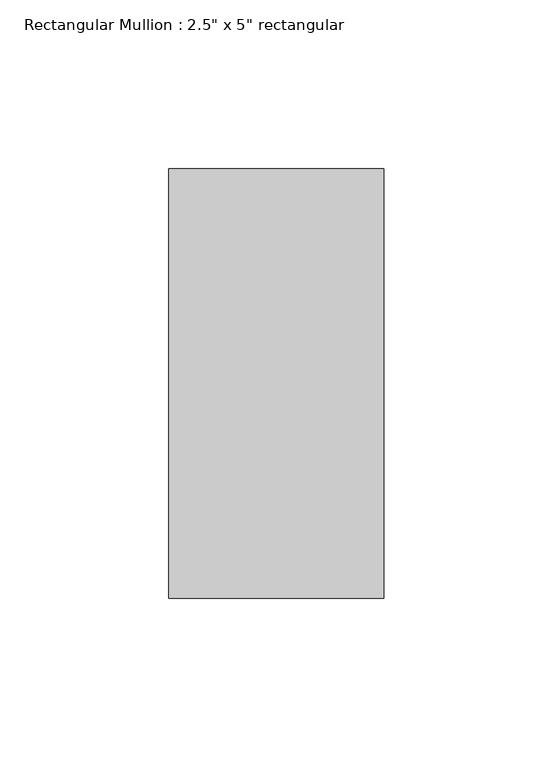
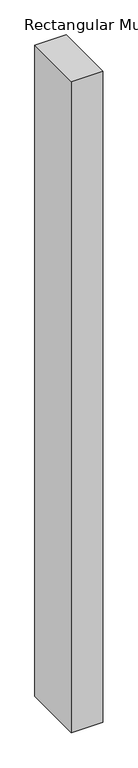
"""IFC4 building model written with IfcOpenShell, lengths in millimetres: member geometry."""

from ifc_helpers import new_model, si_unit, frame, origin, place, context, project, spatial, polyline, outline, extrude, source, transform, mapped, element, save


def member_331a33ef(model_context):
    return source(origin(), model_context, "Body", "SweptSolid", [
        extrude(outline(polyline([(0.0, 63.5), (0.0, -63.5), (-63.5, -63.5), (-63.5, 63.5), (0.0, 63.5)])), frame((0.0, 0.0, -1387.342808), z_axis=(0.0, 0.0, 1.0), x_axis=(1.0, 0.0, 0.0)), (0.0, 0.0, 1.0), 1387.342808),
    ])


if __name__ == "__main__":
    model = new_model("IFC4")
    model_context = context("Model", 3, world=origin())
    ifc_project = project(units=[si_unit("LENGTHUNIT", "METRE", prefix="MILLI")], contexts=[model_context])
    site = spatial("IfcSite", under=ifc_project)
    building = spatial("IfcBuilding", under=site)
    placement = place(None, origin())
    member_shape = member_331a33ef(model_context)
    element("IfcMember", 1, ObjectType="Rectangular Mullion : 2.5\" x 5\" rectangular", at=placement, inside=building, context=model_context, shape_type="MappedRepresentation", body=[
        mapped(member_shape, transform((0.0, 0.0, 0.0), x_axis=(1.0, 0.0, 0.0), y_axis=(0.0, 1.0, 0.0), z_axis=(0.0, 0.0, 1.0))),
    ])
    save(model, "model.ifc")

# Revit data of these elements
# Type "Rectangular Mullion : 2.5\" x 5\" rectangular"
#   built-in parameter 1007304 = 0.416667 (stored number, unit not read)
#   built-in parameter 1007301 = 0.104167 (stored number, unit not read)
#   built-in parameter 1007300 = 0.104167 (stored number, unit not read)
# Element 1 (IfcMember, "Rectangular Mullion : 2.5\" x 5\" rectangular")
#   Materials on its faces: "Aluminum"
# Materials
#   "Aluminum": class "Metal", colour RGB 247 247 247, transparency 0, Description = "Aluminum 6061", Cost = 0
